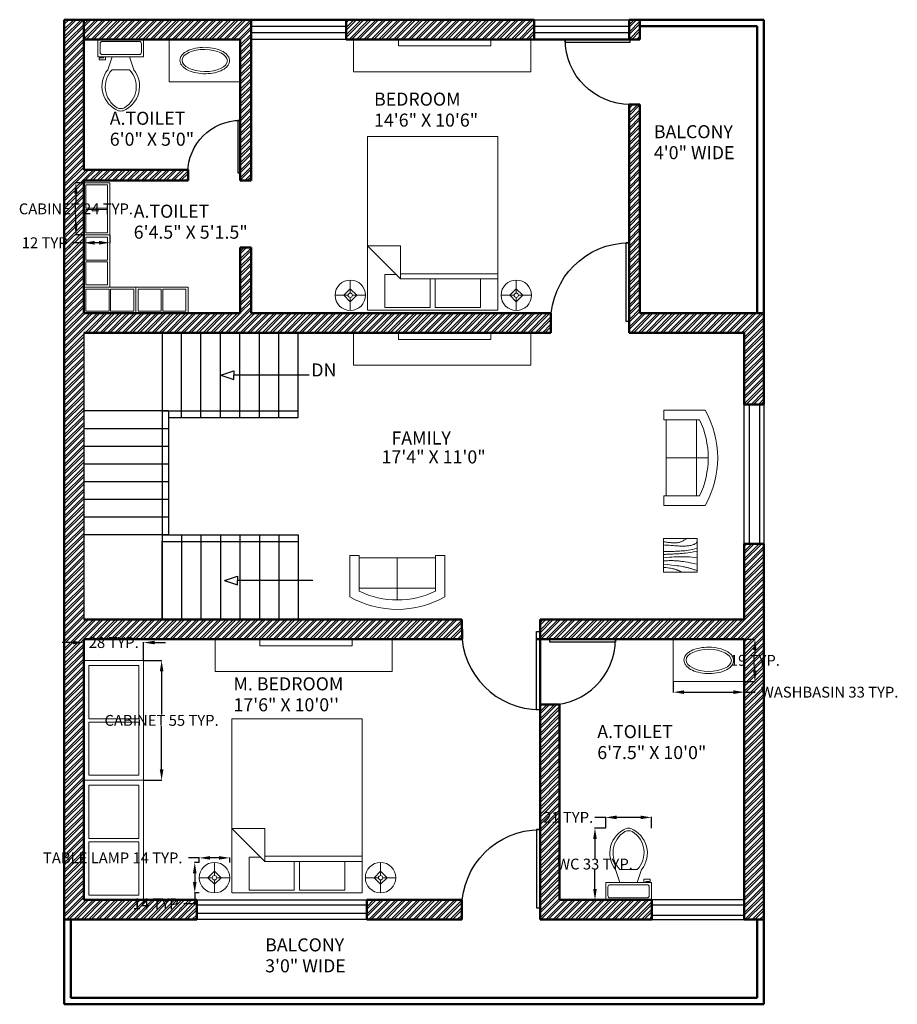
# Model space of a CAD drawing. Units: inches. Extents: x 0 to 822, y 0 to 962.
# Tile 3 of 3: x 418 to 822, y 509 to 962. Entities that reach past the tile are written whole.
import ezdxf

# ---------------------------------------------------------------- set-up
doc = ezdxf.new("R2010")
doc.units = ezdxf.units.IN
doc.header["$MEASUREMENT"] = 0
for name, color, linetype, lineweight in [('A-ANNO-DIMS', 2, 'Continuous', 18), ('A-ANNO-TEXT', 7, 'Continuous', 25), ('A-AREA-IDEN', 7, 'Continuous', 25), ('A-DOOR', 4, 'Continuous', 25), ('A-FLOR-CASE', 5, 'Continuous', 18), ('A-FLOR-FIXT', 8, 'Continuous', 18), ('A-FLOR-STRS', 3, 'Continuous', 25), ('A-FURN', 9, 'Continuous', 18), ('A-GLAZ', 4, 'Continuous', 25), ('A-WALL', 7, 'Continuous', 50), ('A-WALL-PATT', 8, 'Continuous', 13)]:
    doc.layers.add(name, color=color, linetype=linetype, lineweight=lineweight)
doc.styles.get("Standard").update_dxf_attribs({"font": 'arial.ttf'})
doc.dimstyles.get("Standard").update_dxf_attribs({"dimtxt": 5, "dimasz": 5, "dimexe": 0.18, "dimexo": 0.0625, "dimgap": 0.09, "dimtad": 0, "dimtih": 1, "dimtoh": 1, "dimdec": 1, "dimzin": 0, "dimdsep": 46, "dimlunit": 4, "dimtxsty": 'Standard', "dimcen": 0.09, "dimadec": 0, "dimazin": 0, "dimtfac": 1, "dimtdec": 1, "dimtofl": 0, "dimtmove": 0, "dimatfit": 3, "dimfxl": 1, "dimtolj": 1, "dimtzin": 0, "dimarcsym": 0})

# ---------------------------------------------------------------- blocks, each defined once
blk = doc.blocks.new('*U2')
for p, q in [((0, 0), (0, -6)), ((40, 0), (40, -6))]:
    blk.add_line(p, q)
blk.add_lwpolyline([(0, 0), (0, 40), (1.75, 40), (1.75, 0)], close=True)
blk.add_arc((0, 0), 40, 0, 90)
blk = doc.blocks.new('Bed - Queen')
for p, q in [((0, -80.00003), (0, 0)), ((0, 0), (59.99999, 0)), ((59.99999, 0), (59.99999, -80.00003)), ((7.99999, -1.2), (28.79998, -1.2)), ((7.99999, -14.4), (7.99999, -1.2)), ((28.79998, -1.2), (28.79998, -14.4)), ((31.19999, -1.2), (51.99999, -1.2)), ((31.19999, -14.4), (31.19999, -1.2)), ((51.99999, -1.2), (51.99999, -16.4)), ((0, -14.4), (44.8, -14.4)), ((44.8, -16.8), (0, -16.8)), ((59.99999, -29.6), (44.8, -14.4)), ((44.8, -14.4), (44.8, -29.6)), ((51.99999, -16.4), (46.79936, -16.4)), ((44.8, -29.6), (59.99999, -29.6)), ((59.99999, -80.00003), (0, -80.00003))]:
    blk.add_line(p, q)
blk = doc.blocks.new('Lamp - Table')
for p, q in [((0, 7), (0, 1)), ((-1, 0), (-7, 0)), ((0, 3), (-3, 0)), ((-3, 0), (0, -3)), ((3, 0), (0, 3)), ((0, -3), (3, 0)), ((1, 0), (7, 0)), ((0, -1), (0, -7))]:
    blk.add_line(p, q)
for radius in [7, 1]:
    blk.add_circle((0, 0), radius)
blk = doc.blocks.new('Sofa - Roundback Loveseat 5 ft.')
for p, q in [((0, -32.44198), (0, -5.99998)), ((-24, -33.99998), (-24, -11.46958)), ((24.00004, -33.99998), (24.00004, -11.46958)), ((-23.9998, -13.38178), (23.99986, -13.38178)), ((-24, -32.44198), (24.00004, -32.44198))]:
    blk.add_line(p, q)
for points in [[(-24, -33.99998), (-30, -33.99998), (-30, -7.99998)], [(30.00004, -7.99998), (30.00004, -33.99998), (24.00004, -33.99998)]]:
    blk.add_lwpolyline(points)
for centre, radius, start, end in [((0, -60.24998), 60.24998, 60.13715, 119.8628), ((0, -61.38438), 55.38444, 64.32083, 115.6792)]:
    blk.add_arc(centre, radius, start, end)
blk = doc.blocks.new('Table - Square Woodgrain 42 x 42 in.')
blk.add_line((0, -42), (42, -42))
for points in [[(0, -4), (1.704, -4.2172), (3.2358, -4.4188), (4.615, -4.604), (5.8615, -4.7721), (6.9951, -4.9224), (8.0357, -5.0541), (9.0031, -5.1667), (9.9171, -5.2594), (10.7951, -5.3316), (11.6445, -5.3836), (12.4702, -5.4157), (13.277, -5.4283), (14.0698, -5.4217), (14.8535, -5.3964), (15.6331, -5.3526), (16.4133, -5.2908), (17.1986, -5.2103), (17.9913, -5.1062), (18.793, -4.9727), (19.6056, -4.8038), (20.4307, -4.5937), (21.2701, -4.3365), (22.1256, -4.0262), (22.9989, -3.6571), (23.888, -3.2272), (24.7756, -2.7516), (25.6408, -2.2491), (26.4624, -1.7387), (27.2195, -1.2395), (27.891, -0.7703), (28.456, -0.3501), (28.8934, 0.002)], [(0, -42), (0, 0), (42, 0), (42, -42)], [(0, -8), (1.8203, -8.1001), (3.6741, -8.2149), (5.5411, -8.3408), (7.4011, -8.4741), (9.2339, -8.6112), (11.0193, -8.7484), (12.7371, -8.8821), (14.3671, -9.0086), (15.8954, -9.1246), (17.3337, -9.2278), (18.6997, -9.3159), (20.0116, -9.387), (21.2871, -9.4389), (22.5442, -9.4696), (23.8008, -9.477), (25.0749, -9.459), (26.3791, -9.4137), (27.7049, -9.3403), (29.0383, -9.2382), (30.3655, -9.1068), (31.6728, -8.9455), (32.9461, -8.7535), (34.1717, -8.5304), (35.3358, -8.2756), (36.4268, -7.9863), (37.443, -7.6521), (38.3849, -7.2603), (39.253, -6.7986), (40.048, -6.2542), (40.7705, -5.6147), (41.421, -4.8674), (42, -4)], [(42, -12), (39.1784, -12.8621), (36.4519, -13.5654), (33.8246, -14.1294), (31.3004, -14.5731), (28.8832, -14.9161), (26.577, -15.1775), (24.3858, -15.3768), (22.3136, -15.5332), (20.3622, -15.6632), (18.5254, -15.7718), (16.7947, -15.8612), (15.1618, -15.9338), (13.6183, -15.9916), (12.1558, -16.0369), (10.7659, -16.0718), (9.4403, -16.0987), (8.1703, -16.1191), (6.9461, -16.1325), (5.7577, -16.1377), (4.595, -16.1335), (3.4479, -16.1188), (2.3064, -16.0924), (1.1604, -16.0532), (0, -16)], [(42, -16), (37.6529, -16.7365), (33.8802, -17.329), (30.6179, -17.7961), (27.8015, -18.1561), (25.3668, -18.4275), (23.2497, -18.6288), (21.3859, -18.7785), (19.7111, -18.8949), (18.1693, -18.9939), (16.7375, -19.0795), (15.401, -19.1534), (14.1449, -19.217), (12.9544, -19.2717), (11.8148, -19.3191), (10.7113, -19.3606), (9.6291, -19.3976), (8.5534, -19.4323), (7.47, -19.4689), (6.3643, -19.5122), (5.222, -19.5672), (4.0288, -19.6386), (2.7703, -19.7313), (1.4321, -19.8501), (0, -20)], [(0, -24), (3.9243, -23.6805), (7.4766, -23.4138), (10.6891, -23.1954), (13.5943, -23.0205), (16.2247, -22.8847), (18.6125, -22.7832), (20.7903, -22.7116), (22.7903, -22.6651), (24.6563, -22.642), (26.4764, -22.6507), (28.35, -22.7024), (30.3766, -22.8084), (32.6555, -22.98), (35.2861, -23.2283), (38.3678, -23.5645), (42, -24)], [(42, -32), (37.392, -31.017), (33.4585, -30.2231), (30.1291, -29.5949), (27.3334, -29.109), (25.0009, -28.742), (23.0612, -28.4707), (21.4439, -28.2716), (20.0786, -28.1215), (18.8998, -28.0002), (17.8609, -27.9014), (16.9206, -27.8219), (16.0371, -27.7588), (15.1691, -27.709), (14.2748, -27.6693), (13.3128, -27.6368), (12.2415, -27.6083), (11.0295, -27.5824), (9.6867, -27.5643), (8.233, -27.5608), (6.6884, -27.5787), (5.0728, -27.6248), (3.4062, -27.7058), (1.7086, -27.8286), (0, -28)], [(0, -32), (5.4026, -32.5358), (9.9494, -33.019), (13.7424, -33.4553), (16.8834, -33.8505), (19.4743, -34.2106), (21.6171, -34.5413), (23.4136, -34.8486), (24.9657, -35.1382), (26.3614, -35.4156), (27.6332, -35.6841), (28.7995, -35.9467), (29.8788, -36.2064), (30.8897, -36.4661), (31.8507, -36.7288), (32.7802, -36.9973), (33.6968, -37.2747), (34.6175, -37.5635), (35.5531, -37.8651), (36.5128, -38.1805), (37.506, -38.5108), (38.5421, -38.8568), (39.6302, -39.2197), (40.7797, -39.6004), (42, -40)], [(0, -36), (3.0098, -36.2857), (5.5354, -36.5643), (7.6368, -36.8359), (9.374, -37.1009), (10.807, -37.3597), (11.9957, -37.6126), (13.0002, -37.8599), (13.8804, -38.102), (14.6874, -38.3393), (15.4365, -38.5729), (16.1338, -38.8041), (16.7858, -39.0341), (17.3987, -39.264), (17.9787, -39.4952), (18.5322, -39.7288), (19.0655, -39.9662), (19.5832, -40.2081), (20.0842, -40.4544), (20.5657, -40.7046), (21.0249, -40.9581), (21.459, -41.2144), (21.8653, -41.4731), (22.2409, -41.7335), (22.5831, -41.9951)]]:
    blk.add_lwpolyline(points)
blk = doc.blocks.new('Toilet - top')
for p, q in [((9.5, -6), (9.5, -2)), ((-10, -8.5), (-8, -8.5)), ((-10, -9.5), (-10, -8.5)), ((-8, -8.5), (-8, -8)), ((-7, -8), (-7, -9.5)), ((-4, -8), (-6, -14)), ((4, -8), (6, -14)), ((-7, -9.5), (-10, -9.5)), ((4, -14), (-4, -14))]:
    blk.add_line(p, q)
blk.add_lwpolyline([(10.5, -8), (10.5, 0), (-10.5, 0), (-10.5, -8)], close=True)
for points in [[(-9.5, -2), (-9.5, -6)], [(8.5, -1), (-8.5, -1)], [(-8.5, -7), (8.5, -7)]]:
    blk.add_lwpolyline(points)
for centre, radius, start, end in [((-8.62, -1.88), 0.884, 81.8699, 188.1301), ((8.62, -1.88), 0.884, 351.8699, 98.1301), ((-8.62, -6.12), 0.884, 171.8699, 278.1301), ((8.62, -6.12), 0.884, 261.8699, 8.1301), ((3.52, -21.58), 12.17, 141.4691, 247.9714), ((4.2, -21.82), 11.33, 136.3677, 238.9468), ((-3.52, -21.58), 12.17, 292.0284, 38.5307), ((-4.2, -21.82), 11.33, 301.053, 43.6321), ((0, -27.88), 4, 245.7318, 294.2682), ((0, -29), 4, 254.8605, 285.1395)]:
    blk.add_arc(centre, radius, start, end)
blk = doc.blocks.new('Wall Cabinet - 18 x 36 in front')
for p, q in [((17.5, -1.5), (17.5, -16.5)), ((18.5, -16.5), (18.5, -1.5))]:
    blk.add_line(p, q)
blk.add_lwpolyline([(0, -18), (0, 0), (36, 0), (36, -18)], close=True)
for points in [[(17.5, -16.5), (1.5, -16.5), (1.5, -1.5), (17.5, -1.5)], [(18.5, -1.5), (34.5, -1.5), (34.5, -16.5), (18.5, -16.5)]]:
    blk.add_lwpolyline(points)
blk = doc.blocks.new('TV-UNIT')
for points in [[(0, 14.91), (81.55, 14.91), (81.55, 0), (0, 0)], [(20.69, 14.91), (63.1, 14.91), (63.1, 11.87), (20.69, 11.87)]]:
    blk.add_lwpolyline(points, close=True)
blk = doc.blocks.new('WASHBASIN')
blk.add_lwpolyline([(32.67, 19.47), (0, 19.47), (0, 0), (32.67, 0)], close=True)
blk.add_ellipse((16.34, 9.74), major_axis=(-10.4, 0.11), ratio=0.48759)
blk.add_open_spline([(4.94, 9.86), (4.93, 9.45), (5, 9.03), (5.28, 8.24), (5.49, 7.87), (6, 7.17), (6.31, 6.84), (7.45, 5.85), (8.48, 5.28), (10.83, 4.38), (12.16, 4.05), (14.96, 3.67), (16.42, 3.62), (19.28, 3.79), (20.67, 4.02), (23.2, 4.73), (24.33, 5.22), (25.9, 6.24), (26.45, 6.72), (27.19, 7.69), (27.44, 8.15), (27.73, 9.12), (27.77, 9.63), (27.63, 10.63), (27.45, 11.12), (26.93, 12.01), (26.58, 12.42), (25.76, 13.17), (25.28, 13.51), (23.69, 14.44), (22.41, 14.92), (19.6, 15.59), (18.06, 15.78), (14.98, 15.83), (13.44, 15.69), (10.58, 15.12), (9.27, 14.68), (7.35, 13.66), (6.64, 13.15), (5.72, 12.14), (5.41, 11.68), (5.04, 10.77), (4.94, 10.32), (4.94, 9.86)], degree=3, knots=[0, 0, 0, 0, 0.174945, 0.174945, 0.349889, 0.349889, 0.524834, 0.524834, 0.922157, 0.922157, 1.31948, 1.31948, 1.716804, 1.716804, 2.114127, 2.114127, 2.51145, 2.51145, 2.789906, 2.789906, 3.002435, 3.002435, 3.214963, 3.214963, 3.427492, 3.427492, 3.640021, 3.640021, 3.852549, 3.852549, 4.276971, 4.276971, 4.701393, 4.701393, 5.125815, 5.125815, 5.550237, 5.550237, 5.871208, 5.871208, 6.091899, 6.091899, 6.283185, 6.283185, 6.283185, 6.283185])
blk = doc.blocks.new('STAIR-ARROW')
for p, q in [((0, 1.94), (5.97, 3.89)), ((0, 1.94), (5.97, 0)), ((5.97, 3.89), (5.97, 1.94)), ((40.68, 1.94), (5.97, 1.94)), ((5.97, 0), (5.97, 1.94))]:
    blk.add_line(p, q)
blk = doc.blocks.new('*D17')
at = {"layer": 'A-ANNO-DIMS', "color": 0, "lineweight": -2, "transparency": 16777216}
for p, q in [((500.46, 576.31), (495.46, 576.31)), ((500.46, 574.27), (500.46, 576.49)), ((509.46, 576.31), (505.46, 576.31)), ((514.46, 574.27), (514.46, 576.49))]:
    blk.add_line(p, q, dxfattribs=at)
at = {"layer": 'A-ANNO-DIMS', "color": 0, "transparency": 16777216}
for points in [[(505.46, 577.14), (505.46, 575.48), (500.46, 576.31)], [(509.46, 577.14), (509.46, 575.48), (514.46, 576.31)]]:
    blk.add_solid(points, dxfattribs=at)
at = {"layer": 'Defpoints', "color": 0, "transparency": 16777216}
for p in [(500.46, 576.31), (500.46, 574.21), (514.46, 574.21)]:
    blk.add_point(p, dxfattribs=at)
at = {"layer": 'A-ANNO-DIMS', "color": 0, "transparency": 16777216, "insert": (460.62, 576.31), "char_height": 5, "attachment_point": 5}
blk.add_mtext('\\A1;TABLE LAMP 14 TYP.', dxfattribs=at)
blk = doc.blocks.new('*D18')
at = {"layer": 'A-ANNO-DIMS', "color": 0, "lineweight": -2, "transparency": 16777216}
for p, q in [((500.4, 574.21), (498.18, 574.21)), ((498.36, 569.21), (498.36, 565.21)), ((500.4, 560.21), (498.18, 560.21)), ((498.36, 560.21), (498.36, 555.21)), ((498.36, 555.21), (493.36, 555.21))]:
    blk.add_line(p, q, dxfattribs=at)
at = {"layer": 'A-ANNO-DIMS', "color": 0, "transparency": 16777216}
for points in [[(497.53, 569.21), (499.19, 569.21), (498.36, 574.21)], [(497.53, 565.21), (499.19, 565.21), (498.36, 560.21)]]:
    blk.add_solid(points, dxfattribs=at)
at = {"layer": 'Defpoints', "color": 0, "transparency": 16777216}
for p in [(500.46, 574.21), (498.36, 560.21), (500.46, 560.21)]:
    blk.add_point(p, dxfattribs=at)
at = {"layer": 'A-ANNO-DIMS', "color": 0, "transparency": 16777216, "insert": (481.34, 555.21), "char_height": 5, "attachment_point": 5}
blk.add_mtext('\\A1;14 TYP.', dxfattribs=at)
blk = doc.blocks.new('*D19')
at = {"layer": 'A-ANNO-DIMS', "color": 0, "lineweight": -2, "transparency": 16777216}
for p, q in [((447.21, 886.95), (443.49, 886.95)), ((443.67, 881.95), (443.67, 877.62)), ((443.67, 867.95), (443.67, 872.27)), ((447.21, 862.95), (443.49, 862.95))]:
    blk.add_line(p, q, dxfattribs=at)
at = {"layer": 'A-ANNO-DIMS', "color": 0, "transparency": 16777216}
for points in [[(442.84, 881.95), (444.5, 881.95), (443.67, 886.95)], [(442.84, 867.95), (444.5, 867.95), (443.67, 862.95)]]:
    blk.add_solid(points, dxfattribs=at)
at = {"layer": 'Defpoints', "color": 0, "transparency": 16777216}
for p in [(443.67, 886.95), (447.27, 886.95), (447.27, 862.95)]:
    blk.add_point(p, dxfattribs=at)
at = {"layer": 'A-ANNO-DIMS', "color": 0, "transparency": 16777216, "insert": (443.67, 874.95), "char_height": 5, "attachment_point": 5}
blk.add_mtext('\\A1;CABINET 24 TYP.', dxfattribs=at)
blk = doc.blocks.new('*D20')
at = {"layer": 'A-ANNO-DIMS', "color": 0, "lineweight": -2, "transparency": 16777216}
for p, q in [((447.27, 862.88), (447.27, 859.17)), ((459.27, 862.88), (459.27, 859.17)), ((447.27, 859.35), (442.27, 859.35)), ((454.27, 859.35), (452.27, 859.35))]:
    blk.add_line(p, q, dxfattribs=at)
at = {"layer": 'A-ANNO-DIMS', "color": 0, "transparency": 16777216}
for points in [[(452.27, 860.18), (452.27, 858.51), (447.27, 859.35)], [(454.27, 860.18), (454.27, 858.51), (459.27, 859.35)]]:
    blk.add_solid(points, dxfattribs=at)
at = {"layer": 'Defpoints', "color": 0, "transparency": 16777216}
for p in [(447.27, 862.95), (459.27, 862.95), (447.27, 859.35)]:
    blk.add_point(p, dxfattribs=at)
at = {"layer": 'A-ANNO-DIMS', "color": 0, "transparency": 16777216, "insert": (430.25, 859.35), "char_height": 5, "attachment_point": 5}
blk.add_mtext('\\A1;12 TYP.', dxfattribs=at)
blk = doc.blocks.new('*D21')
at = {"layer": 'A-ANNO-DIMS', "color": 0, "lineweight": -2, "transparency": 16777216}
for p, q in [((474.91, 667.12), (483.29, 667.12)), ((483.11, 662.12), (483.11, 642.25)), ((483.11, 617.03), (483.11, 636.9)), ((474.91, 612.03), (483.29, 612.03))]:
    blk.add_line(p, q, dxfattribs=at)
at = {"layer": 'A-ANNO-DIMS', "color": 0, "transparency": 16777216}
for points in [[(482.28, 662.12), (483.95, 662.12), (483.11, 667.12)], [(482.28, 617.03), (483.95, 617.03), (483.11, 612.03)]]:
    blk.add_solid(points, dxfattribs=at)
at = {"layer": 'Defpoints', "color": 0, "transparency": 16777216}
for p in [(474.85, 667.12), (474.85, 612.03), (483.11, 612.03)]:
    blk.add_point(p, dxfattribs=at)
at = {"layer": 'A-ANNO-DIMS', "color": 0, "transparency": 16777216, "insert": (483.11, 639.58), "char_height": 5, "attachment_point": 5}
blk.add_mtext('\\A1;CABINET 55 TYP.', dxfattribs=at)
blk = doc.blocks.new('*D22')
at = {"layer": 'A-ANNO-DIMS', "color": 0, "lineweight": -2, "transparency": 16777216}
for p, q in [((442.31, 675.39), (437.31, 675.39)), ((447.31, 667.19), (447.31, 675.57)), ((474.85, 667.19), (474.85, 675.57)), ((479.85, 675.39), (484.85, 675.39))]:
    blk.add_line(p, q, dxfattribs=at)
at = {"layer": 'A-ANNO-DIMS', "color": 0, "transparency": 16777216}
for points in [[(442.31, 676.22), (442.31, 674.55), (447.31, 675.39)], [(479.85, 676.22), (479.85, 674.55), (474.85, 675.39)]]:
    blk.add_solid(points, dxfattribs=at)
at = {"layer": 'Defpoints', "color": 0, "transparency": 16777216}
for p in [(474.85, 675.39), (447.31, 667.12), (474.85, 667.12)]:
    blk.add_point(p, dxfattribs=at)
at = {"layer": 'A-ANNO-DIMS', "color": 0, "transparency": 16777216, "insert": (461.08, 675.39), "char_height": 5, "attachment_point": 5}
blk.add_mtext('\\A1;28 TYP.', dxfattribs=at)
blk = doc.blocks.new('*D31')
at = {"layer": 'A-ANNO-DIMS', "color": 0, "lineweight": -2, "transparency": 16777216}
for p, q in [((687.49, 589.99), (682.42, 589.99)), ((682.6, 584.99), (682.6, 576.15)), ((682.6, 561.95), (682.6, 570.79)), ((687.49, 556.95), (682.42, 556.95))]:
    blk.add_line(p, q, dxfattribs=at)
at = {"layer": 'A-ANNO-DIMS', "color": 0, "transparency": 16777216}
for points in [[(681.77, 584.99), (683.43, 584.99), (682.6, 589.99)], [(681.77, 561.95), (683.43, 561.95), (682.6, 556.95)]]:
    blk.add_solid(points, dxfattribs=at)
at = {"layer": 'Defpoints', "color": 0, "transparency": 16777216}
for p in [(687.56, 589.99), (682.6, 556.95), (687.56, 556.95)]:
    blk.add_point(p, dxfattribs=at)
at = {"layer": 'A-ANNO-DIMS', "color": 0, "transparency": 16777216, "insert": (682.6, 573.47), "char_height": 5, "attachment_point": 5}
blk.add_mtext('\\A1;WC 33 TYP.', dxfattribs=at)
blk = doc.blocks.new('*D32')
at = {"layer": 'A-ANNO-DIMS', "color": 0, "lineweight": -2, "transparency": 16777216}
for p, q in [((687.56, 594.95), (682.56, 594.95)), ((687.56, 590.05), (687.56, 595.13)), ((703.56, 594.95), (692.56, 594.95)), ((708.56, 590.05), (708.56, 595.13))]:
    blk.add_line(p, q, dxfattribs=at)
at = {"layer": 'A-ANNO-DIMS', "color": 0, "transparency": 16777216}
for points in [[(692.56, 595.78), (692.56, 594.12), (687.56, 594.95)], [(703.56, 595.78), (703.56, 594.12), (708.56, 594.95)]]:
    blk.add_solid(points, dxfattribs=at)
at = {"layer": 'Defpoints', "color": 0, "transparency": 16777216}
for p in [(687.56, 594.95), (687.56, 589.99), (708.56, 589.99)]:
    blk.add_point(p, dxfattribs=at)
at = {"layer": 'A-ANNO-DIMS', "color": 0, "transparency": 16777216, "insert": (670.25, 594.95), "char_height": 5, "attachment_point": 5}
blk.add_mtext('\\A1;21 TYP.', dxfattribs=at)
blk = doc.blocks.new('*D33')
at = {"layer": 'A-ANNO-DIMS', "color": 0, "lineweight": -2, "transparency": 16777216}
for p, q in [((718.63, 657.41), (718.63, 652.39)), ((751.31, 657.41), (751.31, 652.39)), ((723.63, 652.57), (746.31, 652.57)), ((751.31, 652.57), (756.31, 652.57))]:
    blk.add_line(p, q, dxfattribs=at)
at = {"layer": 'A-ANNO-DIMS', "color": 0, "transparency": 16777216}
for points in [[(723.63, 653.41), (723.63, 651.74), (718.63, 652.57)], [(746.31, 653.41), (746.31, 651.74), (751.31, 652.57)]]:
    blk.add_solid(points, dxfattribs=at)
at = {"layer": 'Defpoints', "color": 0, "transparency": 16777216}
for p in [(718.63, 657.47), (751.31, 657.47), (751.31, 652.57)]:
    blk.add_point(p, dxfattribs=at)
at = {"layer": 'A-ANNO-DIMS', "color": 0, "transparency": 16777216, "insert": (790.6, 652.57), "char_height": 5, "attachment_point": 5}
blk.add_mtext('\\A1;WASHBASIN 33 TYP.', dxfattribs=at)
blk = doc.blocks.new('*D34')
at = {"layer": 'A-ANNO-DIMS', "color": 0, "lineweight": -2, "transparency": 16777216}
for p, q in [((751.37, 676.95), (756.39, 676.95)), ((756.21, 671.95), (756.21, 669.85)), ((756.21, 662.47), (756.21, 664.57)), ((751.37, 657.47), (756.39, 657.47))]:
    blk.add_line(p, q, dxfattribs=at)
at = {"layer": 'A-ANNO-DIMS', "color": 0, "transparency": 16777216}
for points in [[(755.37, 671.95), (757.04, 671.95), (756.21, 676.95)], [(755.37, 662.47), (757.04, 662.47), (756.21, 657.47)]]:
    blk.add_solid(points, dxfattribs=at)
at = {"layer": 'Defpoints', "color": 0, "transparency": 16777216}
for p in [(751.31, 676.95), (756.21, 676.95), (751.31, 657.47)]:
    blk.add_point(p, dxfattribs=at)
at = {"layer": 'A-ANNO-DIMS', "color": 0, "transparency": 16777216, "insert": (756.21, 667.21), "char_height": 5, "attachment_point": 5}
blk.add_mtext('\\A1;19 TYP.', dxfattribs=at)

msp = doc.modelspace()

# ---------------------------------------------------------------- hatches: boundary and pattern name
at = {"layer": 'A-WALL-PATT', "transparency": 33554641}
h = msp.add_hatch(dxfattribs=at)
h.set_pattern_fill('ANSI32', color=256, scale=6.4)
h.paths.add_polyline_path([(621.26, 685.95), (447.31, 685.95), (447.31, 817.95), (662.31, 817.95), (662.31, 826.95), (524.31, 826.95), (524.31, 857.14), (519.31, 857.14), (519.31, 826.95), (447.31, 826.95), (447.31, 887.95), (495.31, 887.95), (495.31, 892.95), (447.31, 892.95), (447.31, 961.95), (438.31, 961.95), (438.31, 547.95), (499.26, 547.95), (499.26, 556.95), (447.31, 556.95), (447.31, 676.95), (621.44, 676.95)])
h.paths.add_polyline_path([(666.31, 646.95), (657.31, 646.95), (657.31, 644.49), (657.31, 547.95), (708.81, 547.95), (708.81, 556.95), (666.31, 556.95)], flags=17)
h.paths.add_polyline_path([(760.31, 720.87), (751.31, 720.87), (751.31, 685.95), (657.31, 685.95), (657.31, 680.54), (657.31, 676.95), (751.31, 676.95), (751.31, 547.95), (760.31, 547.95), (760.31, 556.95)])
h.paths.add_polyline_path([(621.31, 556.95), (577.56, 556.95), (577.56, 547.95), (621.31, 547.95)], flags=17)
h.paths.add_polyline_path([(760.31, 817.95), (760.31, 826.95), (703.31, 826.95), (703.31, 922.95), (698.31, 922.95), (698.31, 817.95), (751.31, 817.95), (751.31, 785), (760.31, 785)])
h.paths.add_polyline_path([(654.59, 961.95), (568.02, 961.95), (568.02, 952.95), (654.59, 952.95)])
h.paths.add_polyline_path([(703.31, 961.95), (698.31, 961.95), (698.31, 952.95), (703.31, 952.95)])
h.paths.add_polyline_path([(524.31, 961.95), (447.31, 961.95), (447.31, 952.95), (519.31, 952.95), (519.31, 887.95), (524.31, 887.95)], flags=17)

# ---------------------------------------------------------------- linework, layer by layer
at = {"layer": 'A-FLOR-STRS'}
for p, q in [((447.31, 817.95), (447.31, 685.95)), ((483.31, 817.95), (483.31, 685.95)), ((492.27, 778.95), (492.27, 817.95)), ((501.23, 778.95), (501.23, 817.95)), ((510.19, 778.95), (510.19, 817.95)), ((519.16, 778.95), (519.16, 817.95)), ((528.12, 778.95), (528.12, 817.95)), ((537.08, 778.95), (537.08, 817.95)), ((546.04, 778.95), (546.04, 817.95)), ((486.31, 781.95), (447.31, 781.95)), ((483.31, 781.95), (546.04, 781.95)), ((486.31, 781.95), (486.31, 724.95)), ((486.31, 778.95), (546.04, 778.95)), ((486.31, 773.8), (447.31, 773.8)), ((486.31, 765.66), (447.31, 765.66)), ((486.31, 757.52), (447.31, 757.52)), ((486.31, 749.37), (447.31, 749.37)), ((486.31, 741.23), (447.31, 741.23)), ((486.31, 733.09), (447.31, 733.09)), ((486.31, 724.95), (447.31, 724.95)), ((483.31, 724.95), (546.04, 724.95)), ((492.27, 724.95), (492.27, 685.95)), ((501.23, 724.95), (501.23, 685.95)), ((510.19, 724.95), (510.19, 685.95)), ((519.16, 724.95), (519.16, 685.95)), ((528.12, 724.95), (528.12, 685.95)), ((537.08, 724.95), (537.08, 685.95)), ((546.04, 724.95), (546.04, 685.95)), ((483.31, 685.95), (483.31, 721.95)), ((483.31, 721.95), (546.04, 721.95))]:
    msp.add_line(p, q, dxfattribs=at)
at = {"layer": 'A-GLAZ'}
for points in [[(568.02, 952.9), (524.31, 952.95), (524.31, 961.95), (568.02, 961.9)], [(698.31, 952.95), (654.59, 952.99), (654.59, 961.99), (698.31, 961.95)], [(524.31, 958.98), (568.02, 958.98), (568.02, 955.91), (524.31, 955.91)], [(654.59, 959.02), (698.31, 959.02), (698.31, 955.96), (654.59, 955.96)], [(751.31, 785), (760.31, 785), (760.31, 720.87), (751.31, 720.87)], [(753.73, 785), (758.35, 785), (758.35, 720.87), (753.73, 720.87)], [(499.26, 556.95), (577.56, 556.95), (577.56, 547.95), (499.26, 547.95)], [(499.26, 554.64), (577.56, 554.64), (577.56, 550.67), (499.26, 550.67)], [(751.31, 556.95), (708.81, 556.95), (708.81, 547.95), (751.31, 547.95)], [(708.81, 554.76), (751.31, 554.76), (751.31, 549.82), (708.81, 549.82)]]:
    msp.add_lwpolyline(points, close=True, dxfattribs=at)
at = {"layer": 'A-WALL'}
for p, q in [((438.31, 961.95), (438.31, 547.95)), ((438.31, 961.95), (654.59, 961.95)), ((447.31, 961.95), (447.31, 892.95)), ((524.31, 961.95), (524.31, 887.95)), ((568.02, 961.9), (568.02, 952.95)), ((654.59, 961.99), (654.59, 952.99)), ((698.31, 961.95), (698.31, 952.95)), ((698.31, 961.95), (760.31, 961.95)), ((703.31, 961.95), (703.31, 952.95)), ((760.31, 961.95), (760.31, 817.95)), ((703.31, 958.95), (757.31, 958.95)), ((757.31, 958.95), (757.31, 826.95)), ((447.31, 952.95), (519.31, 952.95)), ((519.31, 952.95), (519.31, 887.95)), ((568.02, 952.95), (698.31, 952.95)), ((698.31, 952.95), (703.31, 952.95)), ((703.31, 922.95), (698.31, 922.95)), ((698.31, 922.95), (698.31, 817.95)), ((703.31, 922.95), (703.31, 826.95)), ((447.31, 892.95), (495.31, 892.95)), ((495.31, 887.95), (495.31, 892.95)), ((447.31, 887.95), (495.31, 887.95)), ((447.31, 887.95), (447.31, 826.95)), ((519.31, 887.95), (524.31, 887.95)), ((519.31, 857.14), (524.31, 857.14)), ((519.31, 857.14), (519.31, 826.95)), ((524.31, 857.14), (524.31, 826.95)), ((447.31, 826.95), (519.31, 826.95)), ((524.31, 826.95), (662.31, 826.95)), ((662.31, 826.95), (662.31, 817.95)), ((703.31, 826.95), (760.31, 826.95)), ((447.31, 817.95), (662.31, 817.95)), ((698.31, 817.95), (751.31, 817.95)), ((751.31, 817.95), (751.31, 785)), ((760.31, 817.95), (760.31, 785)), ((751.31, 785), (760.31, 785)), ((751.31, 720.87), (760.31, 720.87)), ((751.31, 720.87), (751.31, 685.95)), ((760.31, 720.87), (760.31, 556.95)), ((447.31, 685.95), (621.26, 685.95)), ((621.26, 685.95), (621.44, 676.95)), ((657.31, 685.95), (657.31, 547.95)), ((657.31, 685.95), (751.31, 685.95)), ((447.31, 676.95), (621.44, 676.95)), ((447.31, 676.95), (447.31, 556.95)), ((655.73, 676.95), (751.31, 676.95)), ((751.31, 676.95), (751.31, 547.95)), ((666.31, 646.95), (657.31, 646.95)), ((666.31, 646.95), (666.31, 556.95)), ((447.31, 556.95), (499.26, 556.95)), ((499.26, 556.95), (499.26, 547.95)), ((577.56, 556.95), (577.56, 547.95)), ((577.56, 556.95), (621.31, 556.95)), ((621.31, 556.95), (621.31, 547.95)), ((666.31, 556.95), (708.81, 556.95)), ((708.81, 556.95), (708.81, 547.95)), ((760.31, 556.95), (760.31, 508.95)), ((438.31, 547.95), (499.26, 547.95)), ((438.31, 547.95), (438.31, 508.95)), ((441.31, 547.95), (441.31, 511.95)), ((577.56, 547.95), (621.31, 547.95)), ((657.31, 547.95), (708.81, 547.95)), ((751.31, 547.95), (760.31, 547.95)), ((757.31, 547.95), (757.31, 511.95)), ((441.31, 511.95), (757.31, 511.95)), ((438.31, 508.95), (760.31, 508.95))]:
    msp.add_line(p, q, dxfattribs=at)

# ---------------------------------------------------------------- block references
at = {"layer": 'A-DOOR'}
for p, xscale, yscale, zscale, rotation in [((698.82, 952.95), -0.7481725624285693, 0.7481725624285693, 0.7481725624285693, 90), ((657.31, 680.54), 0.9011464770963149, 0.9011464770963149, 0.9011464770963149, 180), ((661.83, 676.95), 0.7538873869804251, 0.7538873869804251, 0.7538873869804251, 270)]:
    msp.add_blockref('*U2', p, dxfattribs=dict(at, xscale=xscale, yscale=yscale, zscale=zscale, rotation=rotation))
for p, xscale, yscale, zscale in [((519.31, 891.56), -0.6023432299022746, 0.6023432299022746, 0.6023432299022746), ((698.31, 823.34), -0.8997116670345121, 0.8997116670345121, 0.8997116670345121), ((657.31, 553.34), -0.8992841812793576, 0.8992841812793576, 0.8992841812793576)]:
    msp.add_blockref('*U2', p, dxfattribs=dict(at, xscale=xscale, yscale=yscale, zscale=zscale))
at = {"layer": 'A-FLOR-CASE'}
for p, xscale, yscale, zscale, rotation in [((447.27, 862.95), 0.6666666666666683, 0.6666666666666683, 0.6666666666666683, 90), ((447.27, 838.95), 0.6666666666666683, 0.6666666666666683, 0.6666666666666683, 90), ((474.85, 667.12), 1.530246656707089, 1.530246656707089, 1.530246656707089, 270), ((474.85, 612.03), 1.530246656707089, 1.530246656707089, 1.530246656707089, 270)]:
    msp.add_blockref('Wall Cabinet - 18 x 36 in front', p, dxfattribs=dict(at, xscale=xscale, yscale=yscale, zscale=zscale, rotation=rotation))
at = {"layer": 'A-FLOR-CASE', "xscale": 0.6666666666666683, "yscale": 0.6666666666666683, "zscale": 0.6666666666666683}
for p in [(447.27, 838.95), (471.27, 838.95)]:
    msp.add_blockref('Wall Cabinet - 18 x 36 in front', p, dxfattribs=at)
at = {"layer": 'A-FLOR-FIXT'}
for name, p in [('Toilet - top', (464.32, 952.95)), ('WASHBASIN', (486.63, 933.47)), ('WASHBASIN', (718.63, 657.47))]:
    msp.add_blockref(name, p, dxfattribs=at)
at = {"layer": 'A-FLOR-FIXT', "rotation": 180}
msp.add_blockref('Toilet - top', (698.06, 556.95), dxfattribs=at)
at = {"layer": 'A-FLOR-STRS'}
for p in [(510.43, 796.5), (512.08, 702)]:
    msp.add_blockref('STAIR-ARROW', p, dxfattribs=at)
at = {"layer": 'A-FURN'}
for p in [(571.51, 938.04), (571.51, 803.04), (507.7, 662.04)]:
    msp.add_blockref('TV-UNIT', p, dxfattribs=at)
at = {"layer": 'A-FURN', "rotation": 180}
for name, p in [('Bed - Queen', (637.88, 828.29)), ('Lamp - Table', (569.96, 835.2)), ('Lamp - Table', (646.39, 835.2)), ('Bed - Queen', (575.38, 560.3)), ('Lamp - Table', (507.46, 567.21)), ('Lamp - Table', (583.9, 567.21))]:
    msp.add_blockref(name, p, dxfattribs=at)
at = {"layer": 'A-FURN', "xscale": 0.730787139360479, "yscale": 0.730787139360479, "zscale": 0.730787139360479}
for p, rotation in [((739.11, 760.37), 270), ((591.61, 690.64), 180)]:
    msp.add_blockref('Sofa - Roundback Loveseat 5 ft.', p, dxfattribs=dict(at, rotation=rotation))
at = {"layer": 'A-FURN', "xscale": 0.3691846535413525, "yscale": 0.3691846535413525, "zscale": 0.3691846535413525}
msp.add_blockref('Table - Square Woodgrain 42 x 42 in.', (714.08, 723.27), dxfattribs=at)

# ---------------------------------------------------------------- texts
at = {"layer": 'A-ANNO-TEXT'}
msp.add_text('DN', height=6, dxfattribs=at).set_placement((552.03, 797.82))
at = {"layer": 'A-AREA-IDEN'}
for s, p in [('BEDROOM', (580.9, 922.43)), ('A.TOILET', (459.25, 913.63)), ('14\'6" X 10\'6"', (580.9, 912.79)), ('BALCONY', (709.71, 907.45)), ('6\'0" X 5\'0"', (459.25, 903.99)), ('4\'0" WIDE', (709.71, 897.81)), ('A.TOILET', (470.27, 870.86)), ('6\'4.5" X 5\'1.5"', (470.27, 861.22)), ('FAMILY', (588.91, 766.52)), ('17\'4" X 11\'0"', (584.36, 757.82)), ('M. BEDROOM', (516.19, 653.4)), ('17\'6" X 10\'0\'\'', (516.19, 643.76)), ('A.TOILET', (683.66, 631.42)), ('6\'7.5" X 10\'0"', (683.66, 621.78)), ('BALCONY', (530.78, 533.29)), ('3\'0" WIDE', (530.78, 523.65))]:
    msp.add_text(s, height=6, dxfattribs=at).set_placement(p)

# ---------------------------------------------------------------- dimensions: what is measured, and where the dimension line sits
at = {"layer": 'A-ANNO-DIMS'}
for base, p1, p2, angle, text, picture, middle in [((443.67, 886.95), (447.27, 862.95), (447.27, 886.95), 90, 'CABINET <> TYP.', '*D19', (443.67, 874.95)), ((447.27, 859.35), (459.27, 862.95), (447.27, 862.95), 180, '<> TYP.', '*D20', (430.25, 859.35)), ((756.21, 676.95), (751.31, 657.47), (751.31, 676.95), 90, '<> TYP.', '*D34', (756.21, 667.21)), ((483.11, 612.03), (474.85, 667.12), (474.85, 612.03), 270, 'CABINET <> TYP.', '*D21', (483.11, 639.58)), ((687.56, 594.95), (708.56, 589.99), (687.56, 589.99), 180, '<> TYP.', '*D32', (670.25, 594.95)), ((500.46, 576.31), (514.46, 574.21), (500.46, 574.21), 180, 'TABLE LAMP <> TYP.', '*D17', (460.62, 576.31)), ((682.6, 556.95), (687.56, 589.99), (687.56, 556.95), 270, 'WC <> TYP.', '*D31', (682.6, 573.47)), ((498.36, 560.21), (500.46, 574.21), (500.46, 560.21), 270, '<> TYP.', '*D18', (481.34, 555.21))]:
    dim = msp.add_linear_dim(base=base, p1=p1, p2=p2, angle=angle, text=text, dimstyle='Standard', override={"dimdec": 0, "dimrnd": 0, "dimzin": 0, "dimlunit": 2}, dxfattribs=at)
    dim.commit()
    dim.dimension.update_dxf_attribs({"geometry": picture, "text_midpoint": middle})
for base, p1, p2, text, picture, middle in [((474.85, 675.39), (447.31, 667.12), (474.85, 667.12), '<> TYP.', '*D22', (461.08, 675.39)), ((751.31, 652.57), (718.63, 657.47), (751.31, 657.47), 'WASHBASIN <> TYP.', '*D33', (790.6, 652.57))]:
    dim = msp.add_linear_dim(base=base, p1=p1, p2=p2, text=text, dimstyle='Standard', override={"dimdec": 0, "dimrnd": 0, "dimzin": 0, "dimlunit": 2}, dxfattribs=at)
    dim.commit()
    dim.dimension.update_dxf_attribs({"geometry": picture, "text_midpoint": middle})

doc.saveas('drawing.dxf')
